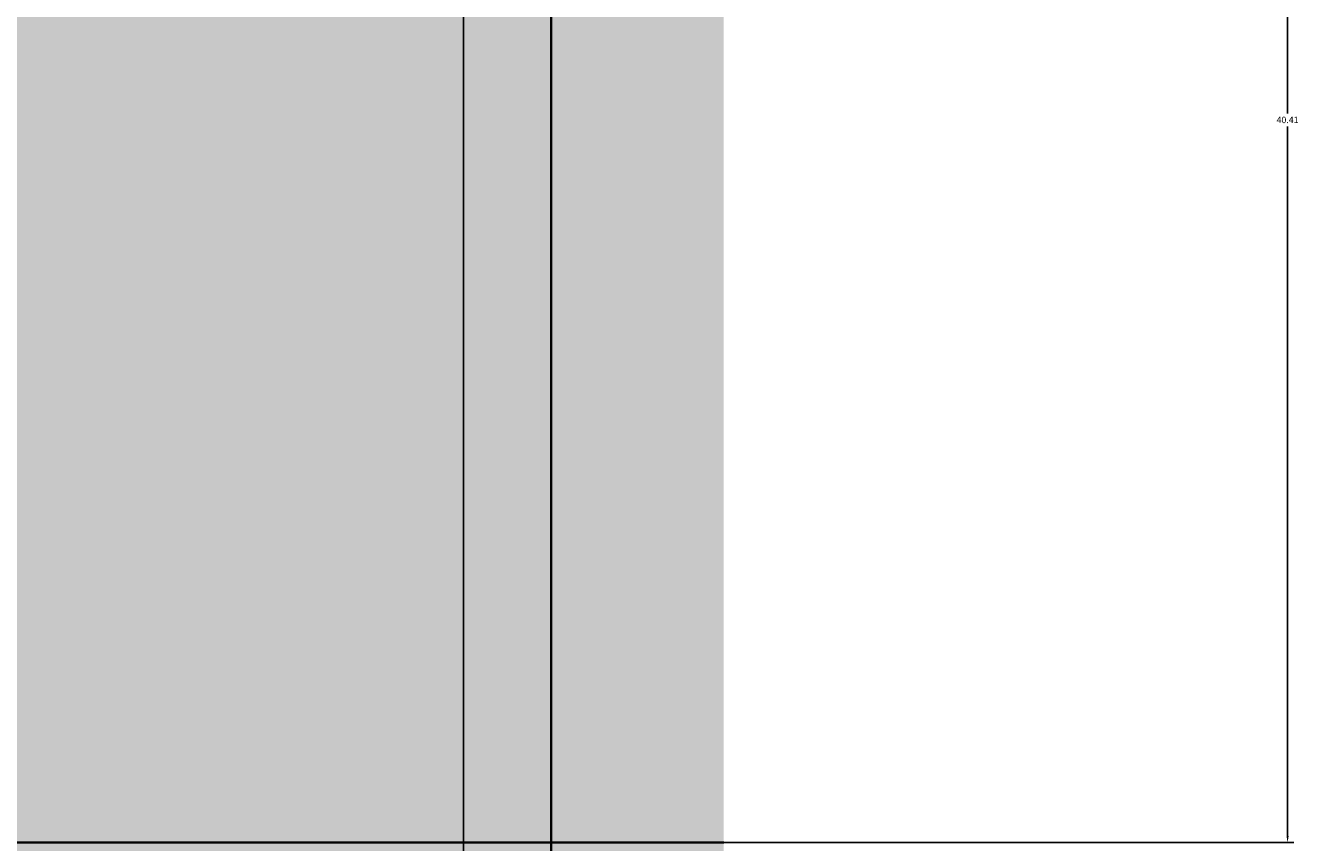
# Model space of a CAD drawing. Units: feet. Extents: x 2695 to 2912, y 795 to 1139.
# Tile 81 of 83: x 2876 to 2912, y 1063 to 1086. Entities that reach past the tile are written whole.
import ezdxf

# ---------------------------------------------------------------- set-up
doc = ezdxf.new("R2010")
doc.units = ezdxf.units.FT
for name, color, linetype, lineweight in [('A-ANNO-DIMS', 2, 'Continuous', 18), ('A-ELEV', 7, 'Continuous', 35), ('A-ELEV-PATT', 252, 'Continuous', 13)]:
    doc.layers.add(name, color=color, linetype=linetype, lineweight=lineweight)
doc.styles.get("Standard").update_dxf_attribs({"font": 'arial.ttf'})
doc.dimstyles.get("Standard").update_dxf_attribs({"dimtxt": 0.18, "dimasz": 0.18, "dimexe": 0.18, "dimexo": 0.0625, "dimgap": 0.09, "dimtad": 0, "dimtih": 1, "dimtoh": 1, "dimdec": 1, "dimzin": 0, "dimdsep": 46, "dimlunit": 3, "dimtxsty": 'Standard', "dimcen": 0.09, "dimadec": 0, "dimazin": 0, "dimtfac": 1, "dimtdec": 1, "dimtofl": 0, "dimtmove": 0, "dimatfit": 3, "dimfxl": 1, "dimtolj": 1, "dimtzin": 0, "dimarcsym": 0})

# ---------------------------------------------------------------- blocks, each defined once
blk = doc.blocks.new('*D11')
at = {"layer": 'A-ANNO-DIMS', "color": 0, "lineweight": -2, "transparency": 16777216}
for p, q in [((2843.575, 1020.886), (2843.575, 1138.886)), ((2895.469, 1107.898), (2895.469, 1138.886)), ((2843.755, 1138.706), (2869.128, 1138.706)), ((2895.289, 1138.706), (2869.916, 1138.706))]:
    blk.add_line(p, q, dxfattribs=at)
at = {"layer": 'A-ANNO-DIMS', "color": 0, "transparency": 16777216}
for points in [[(2843.755, 1138.736), (2843.755, 1138.676), (2843.575, 1138.706)], [(2895.289, 1138.736), (2895.289, 1138.676), (2895.469, 1138.706)]]:
    blk.add_solid(points, dxfattribs=at)
at = {"layer": 'Defpoints', "color": 0, "transparency": 16777216}
for p in [(2895.469, 1138.706), (2895.469, 1107.835), (2843.575, 1020.824)]:
    blk.add_point(p, dxfattribs=at)
at = {"layer": 'A-ANNO-DIMS', "color": 0, "transparency": 16777216, "insert": (2869.522, 1138.706), "char_height": 0.18, "attachment_point": 5}
blk.add_mtext('\\A1;51.89', dxfattribs=at)
blk = doc.blocks.new('*D20')
at = {"layer": 'A-ANNO-DIMS', "color": 0, "lineweight": -2, "transparency": 16777216}
for p, q in [((2895.532, 1103.338), (2911.424, 1103.338)), ((2911.244, 1103.158), (2911.244, 1083.316)), ((2911.244, 1063.111), (2911.244, 1082.952)), ((2890.699, 1062.931), (2911.424, 1062.931))]:
    blk.add_line(p, q, dxfattribs=at)
at = {"layer": 'A-ANNO-DIMS', "color": 0, "transparency": 16777216}
for points in [[(2911.214, 1103.158), (2911.274, 1103.158), (2911.244, 1103.338)], [(2911.214, 1063.111), (2911.274, 1063.111), (2911.244, 1062.931)]]:
    blk.add_solid(points, dxfattribs=at)
at = {"layer": 'Defpoints', "color": 0, "transparency": 16777216}
for p in [(2895.469, 1103.338), (2911.244, 1103.338), (2890.636, 1062.931)]:
    blk.add_point(p, dxfattribs=at)
at = {"layer": 'A-ANNO-DIMS', "color": 0, "transparency": 16777216, "insert": (2911.244, 1083.134), "char_height": 0.18, "attachment_point": 5}
blk.add_mtext('\\A1;40.41', dxfattribs=at)
blk = doc.blocks.new('*D50')
at = {"layer": 'A-ANNO-DIMS', "color": 0, "lineweight": -2, "transparency": 16777216}
for p, q in [((2810.041, 972.03), (2810.041, 1138.886)), ((2888.188, 972.03), (2888.188, 1138.886)), ((2810.221, 1138.706), (2848.721, 1138.706)), ((2888.008, 1138.706), (2849.508, 1138.706))]:
    blk.add_line(p, q, dxfattribs=at)
at = {"layer": 'A-ANNO-DIMS', "color": 0, "transparency": 16777216}
for points in [[(2810.221, 1138.736), (2810.221, 1138.676), (2810.041, 1138.706)], [(2888.008, 1138.736), (2888.008, 1138.676), (2888.188, 1138.706)]]:
    blk.add_solid(points, dxfattribs=at)
at = {"layer": 'Defpoints', "color": 0, "transparency": 16777216}
for p in [(2888.188, 1138.706), (2810.041, 971.967), (2888.188, 971.967)]:
    blk.add_point(p, dxfattribs=at)
at = {"layer": 'A-ANNO-DIMS', "color": 0, "transparency": 16777216, "insert": (2849.114, 1138.706), "char_height": 0.18, "attachment_point": 5}
blk.add_mtext('\\A1;78.15', dxfattribs=at)
blk = doc.blocks.new('*D51')
at = {"layer": 'A-ANNO-DIMS', "color": 0, "lineweight": -2, "transparency": 16777216}
for p, q in [((2888.188, 972.03), (2888.188, 1138.886)), ((2890.636, 972.03), (2890.636, 1138.886)), ((2888.368, 1138.706), (2889.017, 1138.706)), ((2890.456, 1138.706), (2889.808, 1138.706))]:
    blk.add_line(p, q, dxfattribs=at)
at = {"layer": 'A-ANNO-DIMS', "color": 0, "transparency": 16777216}
for points in [[(2888.368, 1138.736), (2888.368, 1138.676), (2888.188, 1138.706)], [(2890.456, 1138.736), (2890.456, 1138.676), (2890.636, 1138.706)]]:
    blk.add_solid(points, dxfattribs=at)
at = {"layer": 'Defpoints', "color": 0, "transparency": 16777216}
for p in [(2890.636, 1138.706), (2888.188, 971.967), (2890.636, 971.967)]:
    blk.add_point(p, dxfattribs=at)
at = {"layer": 'A-ANNO-DIMS', "color": 0, "transparency": 16777216, "insert": (2889.412, 1138.706), "char_height": 0.18, "attachment_point": 5}
blk.add_mtext('\\A1;2.448', dxfattribs=at)

msp = doc.modelspace()

# ---------------------------------------------------------------- hatches: boundary and pattern name
at = {"layer": 'A-ELEV-PATT'}
h = msp.add_hatch(color=256, dxfattribs=at)
h.set_gradient(color1=(255, 255, 255), tint=1)
h.paths.add_polyline_path([(2770.6361, 1122.9306), (2710.6361, 1122.9306), (2710.6361, 1118.4096), (2770.6361, 1118.4096)])
h.paths.add_polyline_path([(2890.6361, 1107.8588), (2770.6361, 1107.8588), (2770.6361, 1103.3378), (2890.6361, 1103.3378)])
h.paths.add_polyline_path([(2890.6361, 1062.9306), (2710.6361, 1062.9306), (2710.6361, 1056.9306), (2710.6361, 936.9306), (2710.6361, 924.3105), (2716.5358, 924.3105), (2890.6361, 924.3105), (2890.6361, 936.9306), (2715.8852, 936.9306), (2715.8852, 1050.3105), (2890.6361, 1050.3105)])
h.paths.add_polyline_path([(2716.5358, 924.3105), (2710.6361, 924.3105), (2710.6361, 810.9306), (2716.5358, 810.9306)])
h = msp.add_hatch(color=256, dxfattribs=at)
h.set_gradient(color1=(147, 149, 152), color2=(147, 149, 152), tint=1)
h.paths.add_polyline_path([(2770.6361, 1118.4096), (2710.6361, 1118.4096), (2710.6361, 1062.9306), (2770.6361, 1062.9306)])
h.paths.add_polyline_path([(2890.6361, 1103.3378), (2770.6361, 1103.3378), (2770.6361, 1062.9306), (2890.6361, 1062.9306)])
h.paths.add_polyline_path([(2730.7081, 1048.1052), (2755.1125, 1048.1052), (2755.1125, 936.9306), (2770.6361, 936.9306), (2770.6361, 1050.3105), (2715.8852, 1050.3105), (2715.8852, 936.9306), (2730.7081, 936.9306)])
h.paths.add_polyline_path([(2890.6361, 1050.3105), (2770.6361, 1050.3105), (2770.6361, 971.9673), (2778.0341, 971.9673), (2778.0341, 1020.8235), (2843.575, 1020.8235), (2843.575, 971.9673), (2890.6361, 971.9673)])
h.paths.add_polyline_path([(2888.1882, 970.7156), (2843.575, 970.7156), (2843.575, 964.8267), (2888.1882, 964.8267)])
h.paths.add_polyline_path([(2888.1882, 964.1328), (2843.575, 964.1328), (2843.575, 956.614), (2888.1882, 956.614)])
h.paths.add_polyline_path([(2888.1882, 955.9202), (2843.575, 955.9202), (2843.575, 949.2892), (2888.1882, 949.2892)])
h.paths.add_polyline_path([(2888.1882, 948.5954), (2843.575, 948.5954), (2843.575, 941.3507), (2888.1882, 941.3507)])
h.paths.add_polyline_path([(2888.1882, 940.6569), (2843.575, 940.6569), (2843.575, 936.9306), (2888.1882, 936.9306)])
h.paths.add_polyline_path([(2890.6361, 970.7156), (2888.9368, 970.7156), (2888.9368, 964.8267), (2890.6361, 964.8267)])
h.paths.add_polyline_path([(2890.6361, 964.1328), (2888.9368, 964.1328), (2888.9368, 956.614), (2890.6361, 956.614)])
h.paths.add_polyline_path([(2890.6361, 955.9202), (2888.9368, 955.9202), (2888.9368, 949.2892), (2890.6361, 949.2892)])
h.paths.add_polyline_path([(2890.6361, 940.6569), (2888.9368, 940.6569), (2888.9368, 936.9306), (2890.6361, 936.9306)])
h.paths.add_polyline_path([(2890.6361, 948.5954), (2888.9368, 948.5954), (2888.9368, 941.3507), (2890.6361, 941.3507)])
h.paths.add_polyline_path([(2772.5216, 970.7156), (2770.6361, 970.7156), (2770.6361, 964.8267), (2772.5216, 964.8267)])
h.paths.add_polyline_path([(2772.5216, 964.1328), (2770.6361, 964.1328), (2770.6361, 956.614), (2772.5216, 956.614)])
h.paths.add_polyline_path([(2772.5216, 955.9202), (2770.6361, 955.9202), (2770.6361, 949.2892), (2772.5216, 949.2892)])
h.paths.add_polyline_path([(2772.5216, 948.5954), (2770.6361, 948.5954), (2770.6361, 941.3507), (2772.5216, 941.3507)])
h.paths.add_polyline_path([(2772.5216, 940.6569), (2770.6361, 940.6569), (2770.6361, 936.9306), (2772.5216, 936.9306)])
h.paths.add_polyline_path([(2778.0341, 940.6569), (2773.2702, 940.6569), (2773.2702, 936.9306), (2778.0341, 936.9306)])
h.paths.add_polyline_path([(2778.0341, 970.7156), (2773.2702, 970.7156), (2773.2702, 964.8267), (2778.0341, 964.8267)])
h.paths.add_polyline_path([(2778.0341, 964.1328), (2773.2702, 964.1328), (2773.2702, 956.614), (2778.0341, 956.614)])
h.paths.add_polyline_path([(2778.0341, 955.9202), (2773.2702, 955.9202), (2773.2702, 949.2892), (2778.0341, 949.2892)])
h.paths.add_polyline_path([(2778.0341, 948.5954), (2773.2702, 948.5954), (2773.2702, 941.3507), (2778.0341, 941.3507)])
h.paths.add_polyline_path([(2810.0407, 940.6569), (2780.0341, 940.6569), (2780.0341, 936.9306), (2810.0407, 936.9306)])
h.paths.add_polyline_path([(2890.6361, 924.3105), (2770.6361, 924.3105), (2770.6361, 810.9306), (2773.5029, 810.9306), (2773.5029, 905.5143), (2805.9398, 905.5143), (2838.3767, 905.5143), (2838.3767, 810.9306), (2890.6361, 810.9306)])
h = msp.add_hatch(color=256, dxfattribs=at)
h.set_gradient(color1=(255, 255, 255), tint=1)
h.paths.add_polyline_path([(2895.4694, 1107.8588), (2890.6361, 1107.8588), (2890.6361, 810.9306), (2895.4694, 810.9306)])
h = msp.add_hatch(color=256, dxfattribs=at)
h.set_gradient(color1=(199, 200, 202), color2=(213, 227, 240), centered=1)
h.paths.add_polyline_path([(2890.6361, 1103.3378), (2770.6361, 1103.3378), (2770.6361, 1062.9306), (2890.6361, 1062.9306)])
h = msp.add_hatch(color=256, dxfattribs=at)
h.set_gradient(color1=(147, 149, 152), color2=(147, 149, 152), tint=1)
h.paths.add_polyline_path([(2895.4694, 1103.3378), (2890.6361, 1103.3378), (2890.6361, 1062.9306), (2895.4694, 1062.9306)])

# ---------------------------------------------------------------- linework, layer by layer
at = {"layer": 'A-ELEV'}
for p, q in [((2890.6361, 810.9306), (2890.6361, 1107.8588)), ((2710.6361, 1062.9306), (2890.6361, 1062.9306)), ((2710.6361, 1062.9306), (2895.4694, 1062.9306)), ((2890.6361, 1062.9306), (2895.4694, 1062.9306)), ((2890.6361, 1062.9306), (2890.6361, 810.9306))]:
    msp.add_line(p, q, dxfattribs=at)

# ---------------------------------------------------------------- dimensions: what is measured, and where the dimension line sits
at = {"layer": 'A-ANNO-DIMS'}
for base, p1, p2, override, picture, middle in [((2888.1882, 1138.7056), (2810.0407, 971.9673), (2888.1882, 971.9673), {"dimdec": 2, "dimlfac": 1, "dimrnd": 0, "dimzin": 0, "dimdsep": 46, "dimlunit": 2}, '*D50', (2849.1144, 1138.7056)), ((2895.4694, 1138.7056), (2843.575, 1020.8235), (2895.4694, 1107.8352), {"dimdec": 2, "dimlfac": 1, "dimrnd": 0, "dimzin": 0, "dimdsep": 46, "dimlunit": 2}, '*D11', (2869.5222, 1138.7056)), ((2890.6361, 1138.7056), (2888.1882, 971.9673), (2890.6361, 971.9673), {"dimdec": 3, "dimlfac": 1, "dimrnd": 0, "dimzin": 0, "dimdsep": 46, "dimlunit": 2}, '*D51', (2889.4121, 1138.7056))]:
    dim = msp.add_linear_dim(base=base, p1=p1, p2=p2, dimstyle='Standard', override=override, dxfattribs=at)
    dim.commit()
    dim.dimension.update_dxf_attribs({"geometry": picture, "text_midpoint": middle})
dim = msp.add_linear_dim(base=(2911.2444, 1103.3378), p1=(2890.6361, 1062.9306), p2=(2895.4694, 1103.3378), angle=90, dimstyle='Standard', override={"dimdec": 2, "dimlfac": 1, "dimrnd": 0, "dimzin": 0, "dimdsep": 46, "dimlunit": 2}, dxfattribs=at)
dim.commit()
dim.dimension.update_dxf_attribs({"geometry": '*D20', "text_midpoint": (2911.2444, 1083.1342)})

doc.saveas('drawing.dxf')
